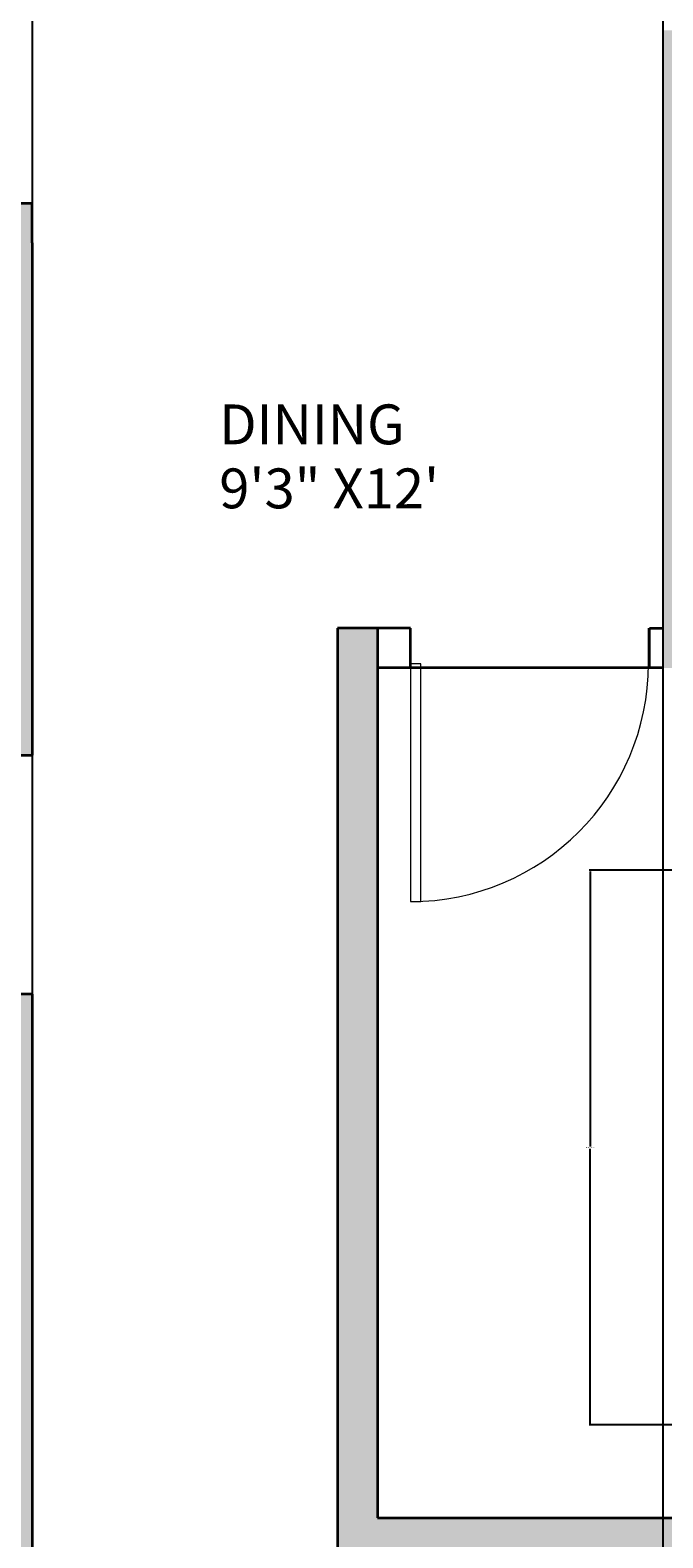
# Model space of a CAD drawing. Units: inches. Extents: x 2070 to 4408, y 1595 to 4269.
# Tile 15 of 20: x 2245 to 2340, y 1949 to 2176. Entities that reach past the tile are written whole.
import ezdxf

# ---------------------------------------------------------------- set-up
doc = ezdxf.new("R2010")
doc.units = ezdxf.units.IN
for name, color, linetype, lineweight in [('A-ANNO-DIMS', 2, 'Continuous', 18), ('A-AREA-IDEN', 7, 'Continuous', 18), ('A-DOOR', 4, 'Continuous', 18), ('A-WALL', 7, 'Continuous', 35)]:
    doc.layers.add(name, color=color, linetype=linetype, lineweight=lineweight)
doc.layers.add('A-WALL-PATT', color=18, linetype='Continuous', lineweight=13, true_color=0x000000)
doc.styles.get("Standard").update_dxf_attribs({"font": 'arial.ttf'})
doc.dimstyles.get("Standard").update_dxf_attribs({"dimtxt": 0.18, "dimasz": 0.18, "dimexe": 0.18, "dimexo": 0.0625, "dimgap": 0.09, "dimtad": 0, "dimtih": 1, "dimtoh": 1, "dimdec": 4, "dimzin": 0, "dimdsep": 46, "dimtxsty": 'Standard', "dimcen": 0.09, "dimadec": 0, "dimazin": 0, "dimtfac": 1, "dimtdec": 4, "dimtofl": 0, "dimtmove": 0, "dimatfit": 3, "dimfxl": 1, "dimtolj": 1, "dimtzin": 0, "dimarcsym": 0})

# ---------------------------------------------------------------- blocks, each defined once
blk = doc.blocks.new('*U3')
for p, q in [((0, 0), (0, 6)), ((40, 0), (40, 6))]:
    blk.add_line(p, q)
blk.add_lwpolyline([(0, 0), (0, -40), (1.75, -40), (1.75, 0)], close=True)
blk.add_arc((0, 0), 40, 270, 0)
blk = doc.blocks.new('*D15')
at = {"layer": 'A-ANNO-DIMS', "color": 0, "lineweight": -2, "transparency": 16777216}
for p, q in [((2341.72, 2049.92), (2329.08, 2049.92)), ((2329.26, 2049.74), (2329.26, 2008.35)), ((2329.26, 1966.6), (2329.26, 2007.99)), ((2341.72, 1966.42), (2329.08, 1966.42))]:
    blk.add_line(p, q, dxfattribs=at)
at = {"layer": 'A-ANNO-DIMS', "color": 0, "transparency": 16777216}
for points in [[(2329.23, 2049.74), (2329.29, 2049.74), (2329.26, 2049.92)], [(2329.23, 1966.6), (2329.29, 1966.6), (2329.26, 1966.42)]]:
    blk.add_solid(points, dxfattribs=at)
at = {"layer": 'Defpoints', "color": 0, "transparency": 16777216}
for p in [(2341.78, 2049.92), (2329.26, 1966.42), (2341.78, 1966.42)]:
    blk.add_point(p, dxfattribs=at)
at = {"layer": 'A-ANNO-DIMS', "color": 0, "transparency": 16777216, "insert": (2329.26, 2008.17), "char_height": 0.18, "attachment_point": 5}
blk.add_mtext('\\A1;BED SET 83', dxfattribs=at)
blk = doc.blocks.new('*D24')
at = {"layer": 'A-ANNO-DIMS', "color": 0, "lineweight": -2, "transparency": 16777216}
for p, q in [((2103.13, 2291.4), (2069.84, 2291.4)), ((2070.02, 2291.22), (2070.02, 1960.08)), ((2070.02, 1628.58), (2070.02, 1959.72)), ((2336.13, 1628.4), (2069.84, 1628.4))]:
    blk.add_line(p, q, dxfattribs=at)
at = {"layer": 'A-ANNO-DIMS', "color": 0, "transparency": 16777216}
for points in [[(2069.99, 2291.22), (2070.05, 2291.22), (2070.02, 2291.4)], [(2069.99, 1628.58), (2070.05, 1628.58), (2070.02, 1628.4)]]:
    blk.add_solid(points, dxfattribs=at)
at = {"layer": 'Defpoints', "color": 0, "transparency": 16777216}
for p in [(2070.02, 2291.4), (2103.2, 2291.4), (2336.2, 1628.4)]:
    blk.add_point(p, dxfattribs=at)
at = {"layer": 'A-ANNO-DIMS', "color": 0, "transparency": 16777216, "insert": (2070.02, 1959.9), "char_height": 0.18, "attachment_point": 5}
blk.add_mtext('\\A1;663', dxfattribs=at)
blk = doc.blocks.new('*D32')
at = {"layer": 'A-ANNO-DIMS', "color": 0, "lineweight": -2, "transparency": 16777216}
for p, q in [((2245.2, 2230.58), (2245.2, 1595.04)), ((2340.2, 2230.58), (2340.2, 1595.04)), ((2245.38, 1595.22), (2292.48, 1595.22)), ((2340.02, 1595.22), (2292.92, 1595.22))]:
    blk.add_line(p, q, dxfattribs=at)
at = {"layer": 'A-ANNO-DIMS', "color": 0, "transparency": 16777216}
for points in [[(2245.38, 1595.25), (2245.38, 1595.19), (2245.2, 1595.22)], [(2340.02, 1595.25), (2340.02, 1595.19), (2340.2, 1595.22)]]:
    blk.add_solid(points, dxfattribs=at)
at = {"layer": 'Defpoints', "color": 0, "transparency": 16777216}
for p in [(2245.2, 2230.65), (2340.2, 2230.65), (2340.2, 1595.22)]:
    blk.add_point(p, dxfattribs=at)
at = {"layer": 'A-ANNO-DIMS', "color": 0, "transparency": 16777216, "insert": (2292.7, 1595.22), "char_height": 0.18, "attachment_point": 5}
blk.add_mtext('\\A1;95', dxfattribs=at)

msp = doc.modelspace()

# ---------------------------------------------------------------- hatches: boundary and pattern name
at = {"layer": 'A-WALL-PATT'}
h = msp.add_hatch(color=256, dxfattribs=at)
h.dxf.hatch_style = 1
h.paths.add_polyline_path([(2346.196, 2218.3995), (2346.196, 2282.3995), (2340.196, 2282.3995), (2340.196, 2212.3995), (2345.5866, 2212.3995), (2346.196, 2212.3995)], flags=0)
h.paths.add_polyline_path([(2245.196, 2282.3995), (2239.196, 2282.3995), (2239.196, 2186.3995), (2244.5866, 2186.3995), (2245.196, 2186.3995)], flags=0)
h.paths.add_polyline_path([(2340.196, 2230.6455), (2245.196, 2230.6455), (2245.196, 2224.6455), (2340.196, 2224.6455)], flags=0)
h.paths.add_polyline_path([(2245.196, 2150.3995), (2239.196, 2150.3995), (2164.4362, 2150.3995), (2164.4362, 2144.3995), (2239.196, 2144.3995), (2239.196, 2086.3995), (2239.196, 2067.2711), (2244.5866, 2067.2711), (2245.196, 2067.2711), (2245.196, 2144.3995)], flags=0)
h.paths.add_polyline_path([(2346.196, 2176.3995), (2340.196, 2176.3995), (2340.196, 2086.3995), (2346.196, 2086.3995), (2346.196, 2125.318)], flags=0)
h.paths.add_polyline_path([(2446.196, 2086.3995), (2346.196, 2086.3995), (2340.196, 2086.3995), (2340.196, 2080.3995), (2446.196, 2080.3995)], flags=0)
h.paths.add_polyline_path([(2455.196, 2291.3995), (2103.196, 2291.3995), (2103.196, 1699.3995), (2336.196, 1699.3995), (2336.196, 1628.3995), (2345.196, 1628.3995), (2446.196, 1628.3995), (2454.8846, 1628.3995), (2454.8846, 1699.3995)])
h.paths.add_polyline_path([(2446.196, 2282.3995), (2446.196, 2218.3995), (2446.196, 2212.3995), (2446.196, 2086.3995), (2446.196, 2080.3995), (2446.196, 1708.3995), (2446.196, 1637.3995), (2345.196, 1637.3995), (2345.196, 1699.3995), (2345.196, 1708.3995), (2336.196, 1708.3995), (2112.196, 1708.3995), (2112.196, 2282.3995), (2239.196, 2282.3995), (2245.196, 2282.3995), (2356.196, 2282.3995)], flags=16)
h.paths.add_polyline_path([(2245.196, 2150.3995), (2245.196, 2144.3995), (2245.196, 2067.2711), (2244.5866, 2067.2711), (2239.196, 2067.2711), (2239.196, 2065.6988), (2203.2929, 2065.6988, 0.40145271), (2239.196, 2031.3337), (2244.5866, 2031.3337), (2245.196, 2031.2711), (2245.196, 1924.1525), (2239.196, 1924.1525), (2239.196, 1922.5803), (2203.2929, 1922.5803, 0.40145271), (2239.196, 1888.2151), (2244.5866, 1888.2151), (2245.196, 1888.1525), (2245.196, 1748.3995), (2339.196, 1748.4621, -0.40145271), (2303.2929, 1782.8272), (2303.2585, 1782.8272), (2303.2585, 1784.3995), (2339.196, 1784.3995), (2339.196, 1877.2067), (2291.196, 1877.2067), (2291.196, 1883.2067), (2291.196, 1946.3995), (2291.196, 1952.3995), (2291.196, 2086.3995), (2297.196, 2086.3995), (2302.196, 2086.3995), (2302.196, 2081.0259), (2303.7633, 2081.0259), (2303.7633, 2080.3995), (2338.0148, 2080.3995, 0.00437129), (2338.0203, 2081.0259), (2338.0203, 2086.3995), (2340.196, 2086.3995), (2340.196, 2176.4621), (2345.5866, 2176.4621, 0.40145271), (2381.4896, 2210.8272), (2345.5866, 2210.8272), (2345.5866, 2212.3995), (2340.196, 2212.3995), (2340.196, 2224.6455), (2245.196, 2224.6455), (2245.196, 2186.3995), (2244.5866, 2186.3995), (2239.196, 2186.3995), (2239.196, 2184.8272), (2203.2929, 2184.8272, 0.40145271), (2239.196, 2150.4621), (2244.5866, 2150.4621)], flags=0)
h.paths.add_polyline_path([(2346.196, 2282.3995), (2346.196, 2218.3995), (2377.1813, 2218.3995), (2377.1813, 2212.3995), (2346.196, 2212.3995), (2345.5866, 2212.3995), (2340.196, 2212.3995), (2340.196, 2224.6455), (2245.196, 2224.6455), (2245.196, 2230.6455), (2245.196, 2282.3995), (2292.696, 2256.5225), (2340.196, 2282.3995)], flags=0)
h.paths.add_polyline_path([(2346.196, 2086.3995), (2340.196, 2086.3995), (2340.196, 2080.3995), (2446.196, 2080.3995), (2431.196, 2016.3995), (2446.196, 1952.3995), (2412.196, 1952.3995), (2412.196, 2080.3995), (2340.196, 2080.3995), (2340.196, 2086.3995), (2340.196, 2176.3995), (2346.196, 2176.3995), (2346.196, 2125.318)], flags=0)
h.paths.add_polyline_path([(2186.508, 2270.0471, -0.03755288), (2186.9712, 2269.8581), (2186.9164, 2270.112, -0.02759121)], flags=0)
h.paths.add_polyline_path([(2183.955, 2273.7766, 1), (2188.2945, 2273.7766, 1)], flags=0)
h.paths.add_polyline_path([(2142.5261, 2274.6158, -0.03707541), (2142.5672, 2275.1696), (2142.5672, 2276.826), (2119.8759, 2276.826), (2119.8759, 2263.0962), (2140.4332, 2263.0962), (2142.5672, 2263.0962), (2142.5672, 2274.0621, -0.03707541)], flags=0)
h.paths.add_polyline_path([(2209.8974, 2263.0962), (2209.8974, 2262.2079), (2190.8042, 2262.2079), (2190.8042, 2263.0962)], flags=0)
h.paths.add_polyline_path([(2210.6382, 2276.1833), (2210.6382, 2263.9844), (2190.2185, 2263.9844), (2190.2185, 2276.1833)], flags=0)
h.paths.add_polyline_path([(2188.4362, 2273.7766, -1), (2183.8133, 2273.7766, -1)], flags=0)
h.paths.add_polyline_path([(2245.196, 2150.3995), (2245.196, 2144.3995), (2245.196, 2067.2711), (2239.196, 2067.2711), (2239.196, 2080.3995), (2172.196, 2080.3995), (2172.196, 2000.3995), (2239.196, 2000.3995), (2239.196, 1940.3995), (2159.0187, 1940.3995), (2123.0187, 1940.3995), (2112.196, 1940.3995), (2112.196, 1946.3995), (2123.0187, 1946.3995), (2123.0187, 1982.2238), (2124.586, 1982.2238), (2124.586, 1982.1895, -0.40145271), (2158.8429, 1946.3995), (2159.0187, 1946.3995), (2239.196, 1946.3995), (2239.196, 1994.3995), (2112.196, 1994.3995), (2112.196, 2000.3995), (2139.196, 2040.3995), (2112.196, 2080.3995), (2112.196, 2086.3995), (2239.196, 2086.3995), (2239.196, 2144.3995), (2209.5809, 2144.3995), (2209.5809, 2136.3995), (2203.0809, 2136.3995), (2205.0809, 2130.3996, -0.70257121), (2199.081, 2116.3995, -0.70256205), (2193.0809, 2130.3994), (2195.0809, 2136.3995), (2192.0809, 2136.3995), (2192.0809, 2134.8995), (2189.0809, 2134.8995), (2189.0809, 2135.8995), (2191.0809, 2135.8995), (2191.0809, 2136.3995), (2188.5809, 2136.3995), (2188.5809, 2144.3995), (2164.2481, 2144.3995, -0.39385849), (2130.0035, 2109.5491), (2130.0035, 2109.5147), (2128.4362, 2109.5147), (2128.4362, 2144.3995), (2112.196, 2144.3995), (2112.196, 2150.3995), (2128.4362, 2150.3995), (2128.4362, 2150.7127), (2164.4362, 2150.7127), (2164.4362, 2150.3995), (2239.196, 2150.3995)], flags=0)
h.paths.add_polyline_path([(2188.2075, 2266.8735), (2188.2075, 2211.8632, -0.41421356), (2185.4833, 2209.1391), (2146.7995, 2209.1391, -0.41421356), (2144.0754, 2211.8632), (2144.0754, 2266.8735, -0.41421356), (2146.7995, 2269.5976), (2185.4833, 2269.5976, -0.41421356)], flags=0)
h.paths.add_polyline_path([(2185.0844, 2273.7766, -1), (2187.1651, 2273.7766, -1)], flags=0)
h.paths.add_polyline_path([(2182.0486, 2259.2932), (2168.0953, 2259.2932), (2168.0953, 2260.8424), (2163.7261, 2260.8424), (2163.7261, 2259.2932), (2149.7727, 2259.2932), (2149.7727, 2266.3352), (2163.7261, 2266.3352), (2163.7261, 2261.9839), (2168.0953, 2261.9839), (2168.0953, 2266.3352), (2182.0486, 2266.3352)], flags=0)
h.paths.add_polyline_path([(2148.2585, 2250.2051), (2153.0615, 2241.8861, 0.39807048)], flags=0)
h.paths.add_polyline_path([(2162.7572, 2247.2885), (2153.1461, 2241.7396), (2148.1083, 2250.4653), (2157.7194, 2256.0142)], flags=0)
h.paths.add_polyline_path([(2162.6726, 2247.4351, -0.39286196), (2157.8415, 2255.6313), (2157.6431, 2255.6313), (2157.8696, 2255.7541)], flags=0)
h.paths.add_polyline_path([(2164.2604, 2145.339), (2164.4362, 2144.3995), (2164.4362, 2150.3995), (2164.2604, 2150.7127)], flags=0)
h.paths.add_polyline_path([(2208.5809, 2142.6495), (2208.5809, 2138.3995, -0.41421356), (2207.8309, 2137.3995), (2190.5809, 2137.3995, -0.41421356), (2189.5809, 2138.1495), (2189.5809, 2142.3995, -0.41421356), (2190.3309, 2143.3995), (2207.5809, 2143.3995, -0.41421356)], flags=0)
h.paths.add_polyline_path([(2147.957, 2229.9119), (2154.7494, 2223.1195, 0.39807048)], flags=0)
h.paths.add_polyline_path([(2162.7165, 2230.8473), (2154.8691, 2222.9998), (2147.7446, 2230.1244), (2155.592, 2237.9718)], flags=0)
h.paths.add_polyline_path([(2162.5969, 2230.9669, -0.39807048), (2155.8044, 2237.7594)], flags=0)
h.paths.add_polyline_path([(2391.8776, 2049.9192), (2408.5766, 2049.9192), (2408.5766, 2033.2202), (2408.5766, 1983.123), (2408.5766, 1966.4239), (2391.8776, 1966.4239), (2391.8776, 1983.123), (2341.7804, 1983.123), (2341.7804, 2033.2202), (2391.8776, 2033.2202)], flags=0)
h.paths.add_polyline_path([(2144.1055, 2274.6158, 1), (2148.445, 2274.6158, 1)], flags=0)
h.paths.add_polyline_path([(2148.5867, 2274.6158, -1), (2143.9638, 2274.6158, -1)], flags=0)
h.paths.add_polyline_path([(2145.2349, 2274.6158, -1), (2147.3156, 2274.6158, -1)], flags=0)
edge = h.paths.add_edge_path(flags=0)
edge.add_ellipse((2400.5951, 2040.9436), major_axis=(-4.5109, 0), ratio=0.97544784, start_angle=180, end_angle=270, ccw=False)
edge.add_ellipse((2400.5951, 2040.9436), major_axis=(-4.5109, 0), ratio=0.97544784, start_angle=90, end_angle=180, ccw=False)
edge.add_ellipse((2400.5951, 2040.9436), major_axis=(-4.5109, 0), ratio=0.97544784, start_angle=0, end_angle=90, ccw=False)
edge.add_ellipse((2400.5951, 2040.9436), major_axis=(-4.5109, 0), ratio=0.97544784, start_angle=270, end_angle=360, ccw=False)
h.paths.add_polyline_path([(2199.0809, 2117.3995, -0.73452973), (2195.0809, 2130.3995), (2203.081, 2130.3995, -0.73453329)], flags=0)
h.paths.add_polyline_path([(2141.9147, 2276.0353), (2141.9147, 2263.9844), (2120.4685, 2263.9844), (2120.4685, 2276.0353)], flags=0)
h.paths.add_polyline_path([(2138.4481, 2273.4072), (2138.4481, 2266.7226), (2133.2801, 2266.7226), (2133.2801, 2273.4072)], flags=0)
h.paths.add_polyline_path([(2137.9691, 2272.9175), (2137.9691, 2272.204), (2135.4229, 2272.204), (2135.4229, 2271.6329), (2135.3221, 2270.1051), (2135.3221, 2269.0265), (2135.4229, 2268.6811), (2135.4229, 2267.2011), (2133.7212, 2267.2011), (2133.7212, 2268.6811), (2133.7983, 2269.9587), (2133.7983, 2271.2758), (2133.7212, 2271.6329), (2133.7212, 2273.0065), (2135.717, 2273.0065), (2135.717, 2272.9175)], flags=0)
h.paths.add_polyline_path([(2137.9215, 2271.8264), (2137.9215, 2271.3786), (2137.5182, 2271.3786), (2136.9355, 2271.3786), (2136.3529, 2271.3786), (2135.7703, 2271.3786), (2135.7703, 2271.8264), (2136.1736, 2271.8264), (2136.7562, 2271.8264), (2137.3389, 2271.8264)], flags=0)
h.paths.add_polyline_path([(2137.9215, 2271.692), (2137.5182, 2271.692), (2136.9355, 2271.513), (2137.3389, 2271.513)], flags=0)
h.paths.add_polyline_path([(2136.3529, 2271.692), (2135.7703, 2271.513), (2136.1736, 2271.513), (2136.7562, 2271.692)], flags=0)
h.paths.add_polyline_path([(2137.9215, 2271.513), (2137.5182, 2271.513), (2136.7562, 2271.747), (2136.7562, 2271.692), (2137.3389, 2271.692)], flags=0)
h.paths.add_polyline_path([(2137.8207, 2270.4664), (2137.8207, 2270.0971), (2137.8207, 2269.627), (2137.8207, 2269.1569), (2137.8207, 2268.6868), (2137.3837, 2268.6868), (2136.6442, 2268.6868), (2135.9271, 2268.6868), (2135.9271, 2269.0562), (2135.9271, 2269.5263), (2135.9271, 2269.9963), (2135.9271, 2270.4664), (2136.3641, 2270.4664), (2137.0812, 2270.4664)], flags=0)
h.paths.add_polyline_path([(2137.3837, 2269.627), (2137.8207, 2269.627), (2137.8207, 2269.5263), (2137.3837, 2269.5263), (2137.3837, 2269.1569), (2137.8207, 2269.1569), (2137.3837, 2269.0562), (2137.3837, 2268.6868), (2137.0812, 2268.6868), (2137.0812, 2269.0562), (2136.6442, 2269.0562), (2136.6442, 2268.6868), (2136.3641, 2268.6868), (2136.3641, 2269.0562), (2135.9271, 2269.0562), (2135.9271, 2269.1569), (2136.3641, 2269.1569), (2136.3641, 2269.5263), (2135.9271, 2269.5263), (2135.9271, 2269.627), (2136.3641, 2269.627), (2136.3641, 2269.9963), (2135.9271, 2269.9963), (2136.3641, 2270.0971), (2136.3641, 2270.4664), (2136.6442, 2270.4664), (2136.6442, 2270.0971), (2137.0812, 2270.0971), (2137.0812, 2270.4664), (2137.3837, 2270.4664), (2137.3837, 2270.0971), (2137.8207, 2270.0971), (2137.3837, 2269.9963)], flags=0)
h.paths.add_polyline_path([(2137.5182, 2271.8264), (2137.5182, 2271.692), (2137.3389, 2271.3786), (2137.3389, 2271.513)], flags=0)
h.paths.add_polyline_path([(2137.8179, 2267.8138), (2137.8179, 2267.6879), (2137.1876, 2267.6879), (2136.4733, 2267.6879), (2135.759, 2267.6879), (2135.759, 2267.8138), (2136.3893, 2267.8138), (2137.1036, 2267.8138)], flags=0)
h.paths.add_polyline_path([(2137.0812, 2269.9963), (2137.0812, 2269.627), (2137.0812, 2269.1569), (2136.6442, 2269.1569), (2136.6442, 2269.5263), (2136.6442, 2269.9963)], flags=0)
h.paths.add_polyline_path([(2136.3529, 2271.8264), (2136.3529, 2271.692), (2136.1736, 2271.3786), (2136.1736, 2271.513)], flags=0)
h.paths.add_polyline_path([(2136.4733, 2267.8138), (2136.4733, 2267.6879), (2136.3893, 2267.6879), (2136.3893, 2267.8138)], flags=0)
h.paths.add_polyline_path([(2407.9087, 2032.5522), (2407.9087, 1983.7909), (2359.81, 1983.7909, -0.00912788), (2359.0575, 1983.7909), (2342.4483, 1983.7909), (2342.4483, 2032.5522)], flags=0)
h.paths.add_polyline_path([(2389.1838, 2023.1358), (2353.7856, 2023.1358), (2353.7856, 1985.4867, -0.09210376), (2350.2788, 1988.655), (2350.2788, 2026.6426), (2389.1838, 2026.6426)], flags=0)
h.paths.add_polyline_path([(2352.6166, 2024.3048), (2351.4477, 2024.3048), (2351.4477, 2025.4737), (2352.6166, 2025.4737)], flags=0)
h.paths.add_polyline_path([(2399.6319, 2026.7589), (2404.3661, 2026.7589, -0.41421356), (2407.0379, 2024.087), (2407.0379, 2013.4908, -0.41421356), (2404.3661, 2010.819), (2399.6319, 2010.819, -0.41421356), (2396.96, 2013.4908), (2396.96, 2024.087, -0.41421356)], flags=0)
h.paths.add_polyline_path([(2399.6319, 2026.0909), (2404.3661, 2026.0909, -0.41421356), (2406.37, 2024.087), (2406.37, 2013.4908, -0.41421356), (2404.3661, 2011.487), (2399.6319, 2011.487, -0.41421356), (2397.628, 2013.4908), (2397.628, 2024.087, -0.41421356)], flags=0)
h.paths.add_polyline_path([(2399.6319, 2002.3217), (2404.3661, 2002.3217, -0.41421356), (2407.0379, 1999.6498), (2407.0379, 1989.0536, -0.41421356), (2404.3661, 1986.3818), (2399.6319, 1986.3818, -0.41421356), (2396.96, 1989.0536), (2396.96, 1999.6498, -0.41421356)], flags=0)
h.paths.add_polyline_path([(2399.6319, 2001.6537), (2404.3661, 2001.6537, -0.41421356), (2406.37, 1999.6498), (2406.37, 1989.0536, -0.41421356), (2404.3661, 1987.0497), (2399.6319, 1987.0497, -0.41421356), (2397.628, 1989.0536), (2397.628, 1999.6498, -0.41421356)], flags=0)
edge = h.paths.add_edge_path(flags=0)
edge.add_ellipse((2400.5951, 1975.3996), major_axis=(-4.5109, 0), ratio=0.97544784, start_angle=-180, end_angle=-90, ccw=False)
edge.add_ellipse((2400.5951, 1975.3996), major_axis=(-4.5109, 0), ratio=0.97544784, start_angle=90, end_angle=180, ccw=False)
edge.add_ellipse((2400.5951, 1975.3996), major_axis=(-4.5109, 0), ratio=0.97544784, start_angle=0, end_angle=90, ccw=False)
edge.add_ellipse((2400.5951, 1975.3996), major_axis=(-4.5109, 0), ratio=0.97544784, start_angle=-90, end_angle=0, ccw=False)
h.paths.add_polyline_path([(2345.196, 1910.3995), (2366.4386, 1910.3995), (2366.4386, 1925.4555), (2392.3856, 1925.4555), (2392.3856, 1933.5025), (2400.1399, 1925.4555), (2392.3856, 1919.8795), (2392.3856, 1925.4555), (2366.4386, 1925.4555), (2366.4386, 1910.3995), (2381.196, 1910.3995), (2405.196, 1910.3995), (2405.196, 1898.3995), (2446.196, 1898.3995), (2446.196, 1886.3995), (2405.196, 1886.3995), (2405.196, 1874.3995), (2446.196, 1874.3995), (2446.196, 1862.3995), (2405.196, 1862.3995), (2405.196, 1850.3995), (2446.196, 1850.3995), (2446.196, 1838.3995), (2405.196, 1838.3995), (2405.196, 1826.3995), (2446.196, 1826.3995), (2446.196, 1814.3995), (2405.196, 1814.3995), (2405.196, 1802.3995), (2446.196, 1802.3995), (2446.196, 1798.3995), (2446.196, 1792.3995), (2405.196, 1792.3995), (2405.196, 1910.3995), (2381.196, 1910.3995), (2381.196, 1792.3995), (2345.196, 1792.3995)], flags=0)
h.paths.add_polyline_path([(2333.0944, 1863.3993, -0.41421356), (2334.7225, 1861.7712), (2334.7225, 1859.329), (2335.2653, 1859.329, -0.41421356), (2337.4361, 1857.1582), (2337.4361, 1843.862, -0.41421356), (2335.2653, 1841.6911, -0.41421356), (2337.4361, 1839.5203), (2337.4361, 1827.5808, -0.41421356), (2335.2653, 1825.41, -0.41421356), (2337.4361, 1823.2392), (2337.4361, 1808.5862, -0.41421356), (2335.2653, 1806.4153), (2334.7225, 1806.4153), (2334.7225, 1803.9732, -0.41421356), (2333.0944, 1802.3451), (2317.356, 1802.3451), (2317.0846, 1802.3451, -0.41421356), (2315.7279, 1803.7018), (2315.7279, 1803.8646), (2313.8284, 1803.8646, -0.41421356), (2311.6576, 1806.0354), (2311.6576, 1823.2015, -0.39597602), (2313.6834, 1825.3765, -0.43384798), (2311.6576, 1827.2718), (2311.6576, 1839.761, -0.41421356), (2313.5571, 1841.6604), (2313.8284, 1841.6604), (2333.8159, 1841.6604, -0.04213623), (2334.1798, 1841.6911, -0.41421356), (2332.009, 1843.862), (2332.009, 1857.1582, -0.41421356), (2334.1798, 1859.329), (2317.356, 1859.329), (2317.0846, 1859.329, -0.41421356), (2315.7279, 1860.6858), (2315.7279, 1862.0426, -0.41421356), (2317.0846, 1863.3993), (2317.356, 1863.3993)], flags=0)
h.paths.add_polyline_path([(2208.8475, 1848.9818), (2208.8475, 1840.9741, -0.41421356), (2207.0458, 1839.1724), (2206.5453, 1839.1721), (2206.5453, 1838.7218, -0.40985861), (2204.7704, 1836.9203), (2183.7501, 1836.9203, -0.41858196), (2181.9216, 1838.7218), (2181.9216, 1839.1721), (2181.421, 1839.1724, -0.41421356), (2179.6193, 1840.9741), (2179.6193, 1848.6817, -0.44064415), (2185.1126, 1854.9874), (2203.3852, 1854.9874, -0.45707961)], flags=0)
h.paths.add_polyline_path([(2204.243, 1848.4815), (2204.243, 1848.4815, 0.41725335), (2202.2204, 1850.4833), (2186.2049, 1850.4833, 0.4111805), (2184.2237, 1848.4815), (2184.2237, 1848.4815, -0.4111807), (2186.2049, 1850.4833), (2202.2204, 1850.4833, -0.41725315)], flags=0)
h.paths.add_polyline_path([(2234.7177, 1830.228), (2234.7176, 1781.6047, -0.41421356), (2233.4381, 1780.3252), (2218.6064, 1780.3252, -0.41421356), (2217.8387, 1781.0929), (2217.8387, 1783.3961, -0.41421356), (2218.6064, 1784.1639), (2218.6065, 1796.9595, -0.41421356), (2219.886, 1798.239, -0.41421356), (2218.6065, 1799.5186), (2218.6065, 1812.3142, -0.41421356), (2219.8861, 1813.5938, -0.41421356), (2218.6065, 1814.8733), (2218.6065, 1827.6689, -0.41421356), (2217.8388, 1828.4367), (2217.8388, 1830.7399, -0.41421356), (2218.6065, 1831.5076), (2233.4382, 1831.5076, -0.41421356)], flags=0)
h.paths.add_polyline_path([(2230.6344, 1827.6689, -0.41421356), (2231.4021, 1826.9012), (2231.4021, 1784.9316, -0.41421356), (2230.6343, 1784.1639), (2221.1853, 1784.1639), (2221.1853, 1827.6689)], flags=0)
h.paths.add_polyline_path([(2222.7208, 1798.239), (2221.6971, 1798.239), (2221.6971, 1813.5938), (2222.7208, 1813.5938)], flags=0)
h.paths.add_polyline_path([(2206.5453, 1773.935), (2206.5453, 1773.4848), (2206.9457, 1773.4848), (2207.0458, 1773.4845, -0.41421356), (2208.8475, 1771.6827), (2208.8475, 1763.675, -0.44222432), (2203.6505, 1757.6695), (2185.3851, 1757.6695, -0.45508402), (2179.6193, 1763.9752), (2179.6193, 1771.6827, -0.41421356), (2181.421, 1773.4845), (2181.421, 1773.4848), (2181.9216, 1773.4848), (2181.9216, 1773.935, -0.40985861), (2183.6965, 1775.7366), (2204.7167, 1775.7366, -0.41858196)], flags=0)
h.paths.add_polyline_path([(2202.2619, 1762.1736), (2186.2464, 1762.1736, -0.41725315), (2184.2237, 1764.1754), (2184.2237, 1764.1754, 0.41725335), (2186.2464, 1762.1736), (2202.2619, 1762.1736, 0.4111805), (2204.243, 1764.1754), (2204.243, 1764.1754, -0.4111807)], flags=0)
h.paths.add_polyline_path([(2313.0034, 1713.1906), (2312.997, 1713.1697), (2313.0123, 1713.1612)], flags=0)
h.paths.add_polyline_path([(2305.7314, 1721.0488), (2305.6257, 1721.1994), (2305.4853, 1721.084)], flags=0)
h.paths.add_polyline_path([(2307.5562, 1726.1427), (2307.6186, 1726.1026), (2307.5737, 1726.0477), (2308.5692, 1720.6434), (2310.5345, 1721.2985), (2310.5721, 1721.411), (2310.6958, 1721.3523), (2313.8453, 1722.4021), (2314.9351, 1723.8033), (2314.9294, 1723.9165), (2315.0028, 1723.8903), (2313.874, 1722.4389), (2313.8697, 1722.4102), (2308.5692, 1720.6434), (2308.9864, 1720.122), (2309.0665, 1720.0971), (2309.053, 1720.0387), (2310.9235, 1717.7005), (2311.4182, 1717.6259), (2311.2918, 1717.2402), (2312.0655, 1716.2731), (2312.1081, 1716.2606), (2312.0969, 1716.2339), (2308.5692, 1720.6434), (2305.2249, 1717.745), (2305.232, 1717.704), (2305.1665, 1717.6944), (2308.5692, 1720.6434)], flags=0)
h.paths.add_polyline_path([(2288.2072, 1714.3431), (2288.2008, 1714.3222), (2288.216, 1714.3137)], flags=0)
h.paths.add_polyline_path([(2280.9352, 1722.2013), (2280.8295, 1722.3519), (2280.689, 1722.2365)], flags=0)
h.paths.add_polyline_path([(2282.76, 1727.2952), (2282.8224, 1727.2551), (2282.7775, 1727.2002), (2283.773, 1721.7959), (2285.7383, 1722.451), (2285.7759, 1722.5635), (2285.8995, 1722.5048), (2289.0491, 1723.5546), (2290.1389, 1724.9558), (2290.1332, 1725.069), (2290.2065, 1725.0428), (2289.0777, 1723.5915), (2289.0735, 1723.5628), (2283.773, 1721.7959), (2284.1901, 1721.2745), (2284.2703, 1721.2496), (2284.2567, 1721.1913), (2286.1273, 1718.8531), (2286.622, 1718.7785), (2286.4956, 1718.3927), (2287.2692, 1717.4256), (2287.3119, 1717.4131), (2287.3006, 1717.3864), (2283.773, 1721.7959), (2280.4286, 1718.8975), (2280.4357, 1718.8565), (2280.3703, 1718.8469), (2283.773, 1721.7959)], flags=0)
h.paths.add_polyline_path([(2302.0672, 1721.8694), (2301.8205, 1721.8572), (2301.7578, 1722.1787), (2299.415, 1724.5215), (2299.103, 1724.4694), (2299.0662, 1724.8703)], flags=0)
h.paths.add_polyline_path([(2264.5643, 1715.4956), (2264.5579, 1715.4747), (2264.5731, 1715.4662)], flags=0)
h.paths.add_polyline_path([(2257.2923, 1723.3538), (2257.1865, 1723.5044), (2257.0461, 1723.389)], flags=0)
h.paths.add_polyline_path([(2259.117, 1728.4477), (2259.1795, 1728.4077), (2259.1345, 1728.3527), (2260.13, 1722.9484), (2262.0954, 1723.6036), (2262.133, 1723.716), (2262.2566, 1723.6573), (2265.4061, 1724.7071), (2266.4959, 1726.1083), (2266.4902, 1726.2215), (2266.5636, 1726.1953), (2265.4348, 1724.744), (2265.4305, 1724.7153), (2260.13, 1722.9484), (2260.5472, 1722.427), (2260.6273, 1722.4022), (2260.6138, 1722.3438), (2262.4843, 1720.0056), (2262.979, 1719.931), (2262.8526, 1719.5452), (2263.6263, 1718.5781), (2263.6689, 1718.5656), (2263.6577, 1718.5389), (2260.13, 1722.9484), (2256.7857, 1720.05), (2256.7928, 1720.009), (2256.7273, 1719.9994), (2260.13, 1722.9484)], flags=0)
h.paths.add_polyline_path([(2277.2709, 1723.0219), (2277.0243, 1723.0097), (2276.9616, 1723.3312), (2274.6187, 1725.6741), (2274.3067, 1725.6219), (2274.27, 1726.0228)], flags=0)
h.paths.add_polyline_path([(2253.628, 1724.1744), (2253.3814, 1724.1622), (2253.3186, 1724.4838), (2250.9758, 1726.8266), (2250.6638, 1726.7744), (2250.627, 1727.1753)], flags=0)
h.paths.add_polyline_path([(2161.9194, 1715.4956), (2161.913, 1715.4747), (2161.9282, 1715.4662)], flags=0)
h.paths.add_polyline_path([(2154.6474, 1723.3538), (2154.5416, 1723.5044), (2154.4012, 1723.389)], flags=0)
h.paths.add_polyline_path([(2162.7899, 1724.744), (2162.7856, 1724.7153), (2157.4851, 1722.9484), (2157.9023, 1722.427), (2157.9824, 1722.4022), (2157.9689, 1722.3438), (2159.8394, 1720.0056), (2160.3341, 1719.931), (2160.2078, 1719.5452), (2160.9814, 1718.5781), (2161.024, 1718.5656), (2161.0128, 1718.5389), (2157.4851, 1722.9484), (2154.1408, 1720.05), (2154.1479, 1720.009), (2154.0824, 1719.9994), (2157.4851, 1722.9484), (2156.4721, 1728.4477), (2156.5346, 1728.4077), (2156.4896, 1728.3527), (2157.4851, 1722.9484), (2159.4505, 1723.6036), (2159.4881, 1723.716), (2159.6117, 1723.6573), (2162.7612, 1724.7071), (2163.851, 1726.1083), (2163.8453, 1726.2215), (2163.9187, 1726.1953)], flags=0)
h.paths.add_polyline_path([(2150.9831, 1724.1744), (2150.7365, 1724.1622), (2150.6738, 1724.4838), (2148.3309, 1726.8266), (2148.0189, 1726.7744), (2147.9822, 1727.1753)], flags=0)
h.paths.add_polyline_path([(2132.5099, 1716.6482), (2132.5035, 1716.6272), (2132.5187, 1716.6187)], flags=0)
h.paths.add_polyline_path([(2125.2379, 1724.5064), (2125.1322, 1724.6569), (2124.9917, 1724.5415)], flags=0)
h.paths.add_polyline_path([(2133.3804, 1725.8965), (2133.3762, 1725.8678), (2128.0757, 1724.101), (2128.4928, 1723.5795), (2128.5729, 1723.5547), (2128.5594, 1723.4963), (2130.43, 1721.1581), (2130.9246, 1721.0835), (2130.7983, 1720.6977), (2131.5719, 1719.7306), (2131.6146, 1719.7181), (2131.6033, 1719.6914), (2128.0757, 1724.101), (2124.7313, 1721.2025), (2124.7384, 1721.1615), (2124.6729, 1721.1519), (2128.0757, 1724.101), (2127.0626, 1729.6002), (2127.1251, 1729.5602), (2127.0801, 1729.5052), (2128.0757, 1724.101), (2130.041, 1724.7561), (2130.0786, 1724.8685), (2130.2022, 1724.8098), (2133.3517, 1725.8597), (2134.4415, 1727.2608), (2134.4358, 1727.3741), (2134.5092, 1727.3478)], flags=0)
h.paths.add_polyline_path([(2121.5736, 1725.3269), (2121.327, 1725.3148), (2121.2643, 1725.6363), (2118.9214, 1727.9791), (2118.6094, 1727.9269), (2118.5727, 1728.3279)], flags=0)
h.paths.add_polyline_path([(2433.3904, 1646.406), (2433.384, 1646.3851), (2433.3992, 1646.3766)], flags=0)
h.paths.add_polyline_path([(2426.1184, 1654.2642), (2426.0127, 1654.4148), (2425.8722, 1654.2994)], flags=0)
h.paths.add_polyline_path([(2427.9432, 1659.3581), (2428.0056, 1659.318), (2427.9606, 1659.2631), (2428.9562, 1653.8588), (2430.9215, 1654.514), (2430.9591, 1654.6264), (2431.0827, 1654.5677), (2434.2323, 1655.6175), (2435.322, 1657.0187), (2435.3163, 1657.1319), (2435.3897, 1657.1057), (2434.2609, 1655.6544), (2434.2567, 1655.6257), (2428.9562, 1653.8588), (2429.3733, 1653.3374), (2429.4534, 1653.3126), (2429.4399, 1653.2542), (2431.3105, 1650.916), (2431.8051, 1650.8414), (2431.6788, 1650.4556), (2432.4524, 1649.4885), (2432.4951, 1649.476), (2432.4838, 1649.4493), (2428.9562, 1653.8588), (2425.6118, 1650.9604), (2425.6189, 1650.9194), (2425.5535, 1650.9098), (2428.9562, 1653.8588)], flags=0)
h.paths.add_polyline_path([(2376.63, 1645.4912), (2376.6236, 1645.4703), (2376.6388, 1645.4617)], flags=0)
h.paths.add_polyline_path([(2369.358, 1653.3494), (2369.2523, 1653.5), (2369.1118, 1653.3845)], flags=0)
h.paths.add_polyline_path([(2371.1828, 1658.4432), (2371.2452, 1658.4032), (2371.2003, 1658.3482), (2372.1958, 1652.944), (2374.1611, 1653.5991), (2374.1987, 1653.7116), (2374.3224, 1653.6528), (2377.4719, 1654.7027), (2378.5617, 1656.1038), (2378.556, 1656.2171), (2378.6293, 1656.1908), (2377.5005, 1654.7395), (2377.4963, 1654.7108), (2372.1958, 1652.944), (2372.6129, 1652.4225), (2372.6931, 1652.3977), (2372.6795, 1652.3393), (2374.5501, 1650.0011), (2375.0448, 1649.9265), (2374.9184, 1649.5407), (2375.692, 1648.5737), (2375.7347, 1648.5611), (2375.7234, 1648.5344), (2372.1958, 1652.944), (2368.8514, 1650.0456), (2368.8586, 1650.0046), (2368.7931, 1649.995), (2372.1958, 1652.944)], flags=0)
h.paths.add_polyline_path([(2404.0947, 1645.0338), (2404.0883, 1645.0128), (2404.1035, 1645.0043)], flags=0)
h.paths.add_polyline_path([(2396.8227, 1652.892), (2396.717, 1653.0425), (2396.5765, 1652.9271)], flags=0)
h.paths.add_polyline_path([(2398.6475, 1657.9858), (2398.7099, 1657.9458), (2398.665, 1657.8908), (2399.6605, 1652.4866), (2401.6258, 1653.1417), (2401.6634, 1653.2541), (2401.7871, 1653.1954), (2404.9366, 1654.2453), (2406.0264, 1655.6464), (2406.0207, 1655.7596), (2406.094, 1655.7334), (2404.9652, 1654.2821), (2404.961, 1654.2534), (2399.6605, 1652.4866), (2400.0776, 1651.9651), (2400.1578, 1651.9403), (2400.1442, 1651.8819), (2402.0148, 1649.5437), (2402.5095, 1649.4691), (2402.3831, 1649.0833), (2403.1567, 1648.1162), (2403.1994, 1648.1037), (2403.1881, 1648.077), (2399.6605, 1652.4866), (2396.3162, 1649.5881), (2396.3233, 1649.5471), (2396.2578, 1649.5375), (2399.6605, 1652.4866)], flags=0)
h.paths.add_polyline_path([(2419.4532, 1658.0857), (2422.4541, 1655.0848), (2422.2075, 1655.0726), (2422.1448, 1655.3941), (2419.8019, 1657.737), (2419.4899, 1657.6848)], flags=0)
h.paths.add_polyline_path([(2390.1575, 1656.7135), (2393.1584, 1653.7125), (2392.9118, 1653.7004), (2392.8491, 1654.0219), (2390.5063, 1656.3647), (2390.1943, 1656.3125)], flags=0)
h.paths.add_polyline_path([(2362.6928, 1657.1709), (2365.6937, 1654.1699), (2365.4471, 1654.1578), (2365.3844, 1654.4793), (2363.0416, 1656.8221), (2362.7295, 1656.77)], flags=0)
h.paths.add_polyline_path([(2419.9523, 2037.8601), (2440.2872, 2037.8601), (2440.2872, 2047.1732), (2419.9523, 2047.1732)], flags=8)
h.paths.add_polyline_path([(2370.186, 1698.9005), (2413.6287, 1698.9005), (2413.6287, 1708.0908), (2370.186, 1708.0908)], flags=8)
h.paths.add_polyline_path([(2370.1656, 1708.5185), (2430.0857, 1708.5185), (2430.0857, 1717.8316), (2370.1656, 1717.8316)], flags=8)
h.paths.add_polyline_path([(2254.1469, 1788.1883), (2302.2471, 1788.1883), (2302.2471, 1797.3786), (2254.1469, 1797.3786)], flags=8)
h.paths.add_polyline_path([(2254.1264, 1797.8063), (2326.1448, 1797.8063), (2326.1448, 1807.1194), (2254.1264, 1807.1194)], flags=8)
h.paths.add_polyline_path([(2300.08, 1914.5069), (2338.861, 1914.5069), (2338.861, 1923.6972), (2300.08, 1923.6972)], flags=8)
h.paths.add_polyline_path([(2300.0595, 1924.1249), (2331.5882, 1924.1249), (2331.5882, 1933.438), (2300.0595, 1933.438)], flags=8)
h.paths.add_polyline_path([(2176.6905, 1716.4567), (2224.1441, 1716.4567), (2224.1441, 1725.647), (2176.6905, 1725.647)], flags=8)
h.paths.add_polyline_path([(2176.67, 1726.0747), (2245.9176, 1726.0747), (2245.9176, 1735.3878), (2176.67, 1735.3878)], flags=8)
h.paths.add_polyline_path([(2339.997, 2039.7696), (2388.1034, 2039.7696), (2388.1034, 2048.9661), (2339.997, 2048.9661)], flags=8)
h.paths.add_polyline_path([(2339.9776, 2049.3928), (2388.7204, 2049.3928), (2388.7204, 2058.7059), (2339.9776, 2058.7059)], flags=8)
h.paths.add_polyline_path([(2366.0063, 2161.3825), (2409.449, 2161.3825), (2409.449, 2170.5728), (2366.0063, 2170.5728)], flags=8)
h.paths.add_polyline_path([(2365.9868, 2171.0016), (2405.879, 2171.0016), (2405.879, 2180.3085), (2365.9868, 2180.3085)], flags=8)
h.paths.add_polyline_path([(2366.0102, 2247.0726), (2407.12, 2247.0726), (2407.12, 2256.263), (2366.0102, 2256.263)], flags=8)
h.paths.add_polyline_path([(2365.9897, 2256.6906), (2397.9686, 2256.6906), (2397.9686, 2266.0037), (2365.9897, 2266.0037)], flags=8)
h.paths.add_polyline_path([(2271.8465, 2102.7885), (2307.6541, 2102.7885), (2307.6541, 2111.9849), (2271.8465, 2111.9849)], flags=8)
h.paths.add_polyline_path([(2271.8281, 2112.4126), (2304.2673, 2112.4126), (2304.2673, 2121.7196), (2271.8281, 2121.7196)], flags=8)
h.paths.add_polyline_path([(2141.6408, 2187.5934), (2182.108, 2187.5934), (2182.108, 2196.7837), (2141.6408, 2196.7837)], flags=8)
h.paths.add_polyline_path([(2141.6203, 2197.2114), (2190.3631, 2197.2114), (2190.3631, 2206.5245), (2141.6203, 2206.5245)], flags=8)
h.paths.add_polyline_path([(2165.7271, 2103.039), (2211.5027, 2103.039), (2211.5027, 2112.2293), (2165.7271, 2112.2293)], flags=8)
h.paths.add_polyline_path([(2165.7077, 2112.658), (2185.1033, 2112.658), (2185.1033, 2121.965), (2165.7077, 2121.965)], flags=8)
h.paths.add_polyline_path([(2174.945, 2048.0789), (2211.3973, 2048.0789), (2211.3973, 2057.2693), (2174.945, 2057.2693)], flags=8)
h.paths.add_polyline_path([(2174.9256, 2057.698), (2194.3212, 2057.698), (2194.3212, 2067.0049), (2174.9256, 2067.0049)], flags=8)
h.paths.add_polyline_path([(2164.8305, 1965.8394), (2202.9649, 1965.8394), (2202.9649, 1975.0297), (2164.8305, 1975.0297)], flags=8)
h.paths.add_polyline_path([(2164.8111, 1975.4584), (2184.2067, 1975.4584), (2184.2067, 1984.7654), (2164.8111, 1984.7654)], flags=8)
h.paths.add_polyline_path([(2133.0392, 1862.086), (2173.5065, 1862.086), (2173.5065, 1871.2763), (2133.0392, 1871.2763)], flags=8)
h.paths.add_polyline_path([(2133.0709, 1871.8585), (2157.0382, 1871.8585), (2157.0382, 1880.8585), (2133.0709, 1880.8585)], flags=8)
h.paths.add_polyline_path([(2406.4423, 1923.5541), (2418.8209, 1923.5541), (2418.8209, 1932.7199), (2406.4423, 1932.7199)], flags=8)
h = msp.add_hatch(color=256, dxfattribs=at)
h.dxf.hatch_style = 1
h.paths.add_polyline_path([(2245.196, 2282.3995), (2239.196, 2282.3995), (2239.196, 2186.3995), (2244.5866, 2186.3995), (2245.196, 2186.3995)])
h.paths.add_polyline_path([(2340.196, 2230.6455), (2245.196, 2230.6455), (2245.196, 2224.6455), (2340.196, 2224.6455)])
h.paths.add_polyline_path([(2346.196, 2282.3995), (2340.196, 2282.3995), (2340.196, 2212.3995), (2345.5866, 2212.3995), (2346.196, 2212.3995), (2346.196, 2218.3995)])
h.paths.add_polyline_path([(2245.196, 2144.3995), (2245.196, 2150.3995), (2239.196, 2150.3995), (2164.4362, 2150.3995), (2164.4362, 2144.3995), (2239.196, 2144.3995), (2239.196, 2086.3995), (2239.196, 2067.2711), (2244.5866, 2067.2711), (2245.196, 2067.2711)])
h.paths.add_polyline_path([(2128.4362, 2150.3995), (2112.196, 2150.3995), (2112.196, 2144.3995), (2128.4362, 2144.3995), (2128.4362, 2145.339)])
h.paths.add_polyline_path([(2239.196, 2086.3995), (2112.196, 2086.3995), (2112.196, 2080.3995), (2239.196, 2080.3995)])
h.paths.add_polyline_path([(2172.196, 2080.3995), (2166.196, 2080.3995), (2166.196, 2000.3995), (2172.196, 2000.3995)])
h.paths.add_polyline_path([(2239.196, 2000.3995), (2112.196, 2000.3995), (2112.196, 1994.3995), (2239.196, 1994.3995)])
h.paths.add_polyline_path([(2245.196, 2031.2711), (2239.196, 2031.2711), (2239.196, 2000.3995), (2239.196, 1940.3995), (2245.196, 1940.3995)])
h.paths.add_polyline_path([(2239.196, 1946.3995), (2159.0187, 1946.3995), (2159.0187, 1940.3995), (2239.196, 1940.3995)])
h.paths.add_polyline_path([(2123.0187, 1946.3995), (2112.196, 1946.3995), (2112.196, 1940.3995), (2123.0187, 1940.3995)])
h.paths.add_polyline_path([(2377.1813, 2218.3995), (2346.196, 2218.3995), (2346.196, 2212.3995), (2377.1813, 2212.3995)])
h.paths.add_polyline_path([(2446.196, 2218.3995), (2413.1813, 2218.3995), (2413.1813, 2212.3995), (2446.196, 2212.3995)])
h.paths.add_polyline_path([(2446.196, 2086.3995), (2346.196, 2086.3995), (2340.196, 2086.3995), (2340.196, 2080.3995), (2446.196, 2080.3995)], flags=17)
h.paths.add_polyline_path([(2346.196, 2125.318), (2346.196, 2176.3995), (2340.196, 2176.3995), (2340.196, 2086.3995), (2346.196, 2086.3995)])
h.paths.add_polyline_path([(2245.196, 1888.1525), (2239.196, 1888.1525), (2239.196, 1748.3995), (2245.196, 1748.3995)])
h.paths.add_polyline_path([(2345.196, 1748.3995), (2239.196, 1748.3995), (2112.196, 1748.3995), (2112.196, 1742.3995), (2239.196, 1742.3995), (2345.196, 1742.3995)])
h.paths.add_polyline_path([(2297.196, 2080.3995), (2297.196, 2086.3995), (2291.196, 2086.3995), (2291.196, 1952.3995), (2291.196, 1946.3995), (2339.196, 1946.3995), (2339.196, 1883.2067), (2291.196, 1883.2067), (2291.196, 1877.2067), (2339.196, 1877.2067), (2339.196, 1784.3995), (2345.196, 1784.3995), (2345.196, 1792.3995), (2345.196, 1946.3995), (2446.196, 1946.3995), (2446.196, 1952.3995), (2297.196, 1952.3995)])

# ---------------------------------------------------------------- linework, layer by layer
at = {"layer": 'A-WALL'}
for p, q in [((2239.196, 2150.3995), (2245.196, 2150.3995)), ((2245.196, 2144.3995), (2245.196, 2150.3995)), ((2245.196, 2144.3995), (2245.196, 2067.2711)), ((2297.196, 2086.3995), (2291.196, 2086.3995)), ((2291.196, 2086.3995), (2291.196, 1952.3995)), ((2302.196, 2086.3995), (2297.196, 2086.3995)), ((2297.196, 2086.3995), (2297.196, 2080.3995)), ((2302.196, 2080.3995), (2302.196, 2086.3995)), ((2338.196, 2080.3995), (2338.196, 2086.3995)), ((2338.196, 2086.3995), (2340.196, 2086.3995)), ((2297.196, 2080.3995), (2297.196, 1952.3995)), ((2302.196, 2080.3995), (2297.196, 2080.3995)), ((2338.196, 2080.3995), (2302.196, 2080.3995)), ((2340.196, 2080.3995), (2338.196, 2080.3995)), ((2239.196, 2067.2711), (2245.196, 2067.2711)), ((2245.196, 2031.2711), (2239.196, 2031.2711)), ((2245.196, 2031.2711), (2245.196, 1924.1525)), ((2291.196, 1952.3995), (2291.196, 1946.3995)), ((2297.196, 1952.3995), (2446.196, 1952.3995))]:
    msp.add_line(p, q, dxfattribs=at)

# ---------------------------------------------------------------- block references
at = {"layer": 'A-DOOR', "xscale": 0.8956071672485885, "yscale": 0.8956071672485885, "zscale": 0.8956071672485885}
msp.add_blockref('*U3', (2302.196, 2081.0259), dxfattribs=at)

# ---------------------------------------------------------------- texts
at = {"layer": 'A-AREA-IDEN'}
for s, p in [('DINING', (2273.3792, 2114.0661)), ('9\'3" X12\'', (2273.3792, 2104.4276))]:
    msp.add_text(s, height=6, dxfattribs=at).set_placement(p)

# ---------------------------------------------------------------- dimensions: what is measured, and where the dimension line sits
at = {"layer": 'A-ANNO-DIMS'}
dim = msp.add_linear_dim(base=(2070.016, 2291.3995), p1=(2336.196, 1628.3995), p2=(2103.196, 2291.3995), angle=90, dimstyle='Standard', override={"dimdec": 0, "dimlfac": 1, "dimrnd": 0, "dimzin": 0, "dimdsep": 46, "dimlunit": 2}, dxfattribs=at)
dim.commit()
dim.dimension.update_dxf_attribs({"geometry": '*D24', "text_midpoint": (2070.016, 1959.8995)})
dim = msp.add_linear_dim(base=(2340.196, 1595.2195), p1=(2245.196, 2230.6455), p2=(2340.196, 2230.6455), dimstyle='Standard', override={"dimdec": 0, "dimlfac": 1, "dimrnd": 0, "dimzin": 0, "dimdsep": 46, "dimlunit": 2}, dxfattribs=at)
dim.commit()
dim.dimension.update_dxf_attribs({"geometry": '*D32', "text_midpoint": (2292.696, 1595.2195)})
dim = msp.add_linear_dim(base=(2329.2561, 1966.4239), p1=(2341.7804, 2049.9192), p2=(2341.7804, 1966.4239), angle=270, text='BED SET <>', dimstyle='Standard', override={"dimdec": 0, "dimlfac": 1, "dimrnd": 0, "dimzin": 0, "dimdsep": 46, "dimlunit": 2}, dxfattribs=at)
dim.commit()
dim.dimension.update_dxf_attribs({"geometry": '*D15', "text_midpoint": (2329.2561, 2008.1716)})

doc.saveas('drawing.dxf')
